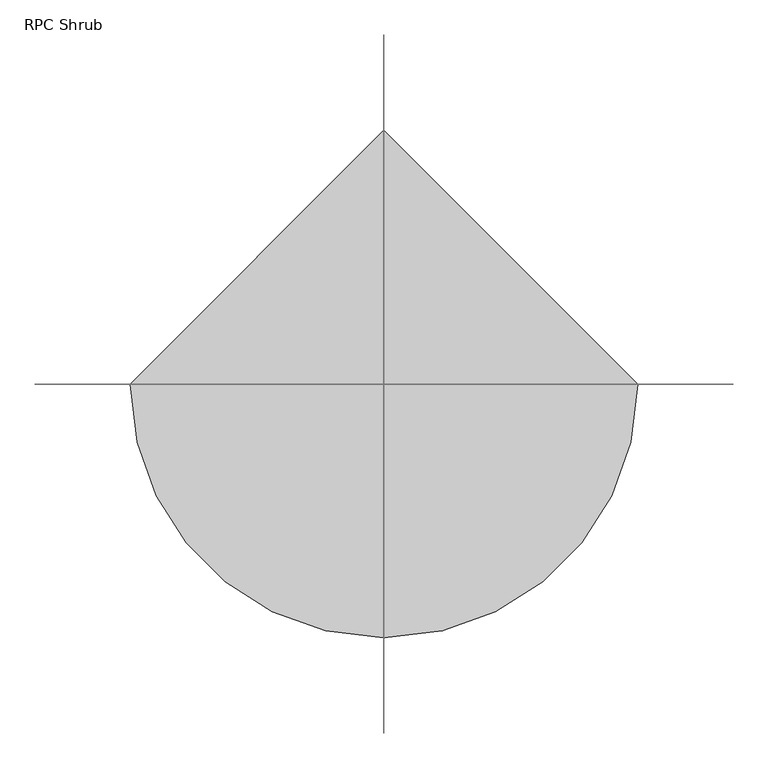
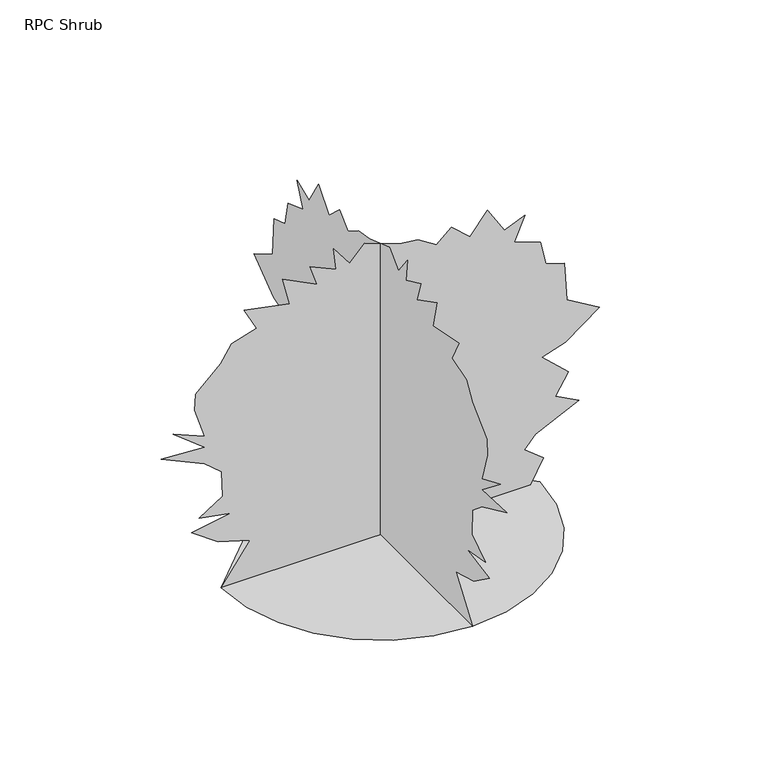
"""IFC4 building model written with IfcOpenShell, lengths in millimetres: geographic element geometry, RPC Shrub."""

from ifc_helpers import new_model, si_unit, origin, place, context, project, spatial, triangles, source, transform, mapped, element, save


def rpc_shrub_d2795376(model_context):
    return source(origin(), model_context, "Body", "Tessellation", [
        triangles([(-812.5409557, 0.0, 3.62e-05), (-791.0601448, -186.180478, 3.62e-05), (-729.8816843, -357.1570149, 3.62e-05), (-633.9078186, -508.0330164, 3.62e-05), (-508.0330164, -633.9078186, 3.62e-05), (-357.1570149, -729.8816843, 3.62e-05), (-186.180478, -791.0601448, 3.62e-05), (3.55e-05, -812.5409557, 3.62e-05), (186.180478, -791.0601448, 3.62e-05), (357.1570149, -729.8816843, 3.62e-05), (508.0330164, -633.9078186, 3.62e-05), (633.9078186, -508.0330164, 3.62e-05), (729.8816843, -357.1570149, 3.62e-05), (791.0601448, -186.180478, 3.62e-05), (812.5409557, 7.1e-05, 3.62e-05), (-0.0001066, 812.5409557, 3.62e-05), (-0.0042747, -811.2988804, 0.0001209), (-0.0042708, -665.7314575, 204.5081021), (-0.004267, -827.9002653, 251.4511125), (-0.004262, -964.4608252, 349.6055863), (-0.004264, -763.884696, 383.7457263), (-0.0042607, -926.0535038, 413.6186849), (-0.0042602, -806.5617422, 490.4333639), (-0.0042562, -810.8289963, 622.7267424), (-0.0042527, -896.1805452, 695.2767471), (-0.0042464, -1118.0927267, 797.697167), (-0.0042501, -896.1805452, 784.8930067), (-0.0042438, -1058.3468822, 912.9192038), (-0.0042483, -896.1805452, 844.6389238), (-0.0042428, -947.3895561, 1002.5380068), (-0.0042404, -943.1223021, 1087.8896284), (-0.0042387, -815.0961777, 1207.38139), (-0.0042368, -759.6175146, 1297.000193), (-0.0042376, -631.5913176, 1335.4075871), (-0.0042331, -695.6044161, 1454.899276), (-0.0042379, -465.1578355, 1407.9550484), (-0.0042331, -499.2979754, 1553.0525871), (-0.0042384, -324.3300579, 1463.4336388), (-0.0042347, -358.4701979, 1570.1213127), (-0.0042384, -226.1755659, 1510.3753956), (-0.0042348, -238.9781819, 1625.6000484), (-0.0042392, -157.8947773, 1518.9123745), (-0.0042379, -81.0790899, 1599.9941986), (-0.0042425, 98.1577894, 1535.9812454), (-0.0042443, 192.0433106, 1523.1795559), (-0.0042475, 285.9303487, 1463.4336388), (-0.0042466, 362.7450096, 1531.7139187), (-0.0042505, 456.6310304, 1446.3622971), (-0.0042486, 546.2498697, 1557.3197685), (-0.0042539, 631.6014914, 1420.7592087), (-0.0042542, 738.2890926, 1463.4336388), (-0.0042571, 682.8104296, 1339.6747684), (-0.0042604, 815.1063515, 1292.7303955), (-0.0042647, 844.9766939, 1164.7042711), (-0.004267, 938.862751, 1134.8313852), (-0.0042731, 951.6669113, 934.2577269), (-0.0042786, 1118.1003571, 836.1044884), (-0.0042798, 943.1324759, 708.078364), (-0.0042791, 823.6407143, 669.67097), (-0.004285, 960.2012741, 541.6448456), (-0.0042871, 891.9209942, 434.9546645), (-0.0042908, 1011.4127558, 370.9416023), (-0.0042907, 789.5005743, 264.2539829), (-0.0042918, 734.0219112, 200.2406482), (-0.0042955, 832.1751497, 123.4246974), (-0.0042982, 766.4170269, 0.0205859), (-811.3090542, 0.0043453, 0.0), (-665.7416313, 0.0043331, 204.5081021), (-827.9078957, 0.0043303, 251.4511125), (-964.4684555, 0.0043245, 349.6055863), (-763.8948698, 0.0043224, 383.7457263), (-926.0611341, 0.0043206, 413.6186849), (-806.5693726, 0.0043161, 490.4333639), (-810.836554, 0.0043082, 622.7267424), (-896.1881756, 0.0043039, 695.2742037), (-1118.1003571, 0.0042978, 797.697167), (-896.1881756, 0.0042985, 784.8930067), (-1058.3545126, 0.0042909, 912.9192038), (-896.1881756, 0.004295, 844.6389238), (-947.3996572, 0.0042855, 1002.5380068), (-943.1299324, 0.0042805, 1087.8896284), (-815.1063515, 0.0042733, 1207.38139), (-759.6276157, 0.004268, 1297.000193), (-631.6014914, 0.0042657, 1335.4075871), (-695.6145899, 0.0042586, 1454.899276), (-465.1654295, 0.0042614, 1407.9550484), (-499.3055695, 0.0042527, 1553.0525871), (-324.3376883, 0.0042581, 1463.4336388), (-358.4778282, 0.0042517, 1570.1213127), (-226.1839592, 0.0042553, 1510.3753956), (-238.9868297, 0.0042484, 1625.6000484), (-157.903425, 0.0042548, 1518.9123745), (-81.0877195, 0.0042499, 1599.9941986), (98.1491599, 0.0042537, 1535.9812454), (192.0346629, 0.0042545, 1523.1795559), (285.9201749, 0.0042581, 1463.4336388), (362.7374156, 0.004254, 1531.7139187), (456.6234364, 0.0042591, 1446.3622971), (546.2422394, 0.0042525, 1557.3197685), (631.5913176, 0.0042606, 1420.7565926), (738.2814623, 0.0042581, 1463.4336388), (682.8027992, 0.0042654, 1339.6747684), (815.0961777, 0.0042682, 1292.7303955), (844.9691362, 0.0042759, 1164.7042711), (938.8551207, 0.0042777, 1134.8313852), (951.6567375, 0.0042896, 934.2577269), (1118.0927267, 0.0042955, 836.1044884), (943.1223021, 0.0043031, 708.078364), (823.6305405, 0.0043054, 669.67097), (960.1936438, 0.004313, 541.6448456), (891.9133638, 0.0043194, 434.9546645), (1011.402582, 0.0043232, 370.9416023), (789.4904005, 0.0043296, 264.2539829), (734.0142809, 0.0043334, 200.2403938), (832.1675194, 0.0043379, 123.4246974), (766.4094692, 0.0043453, 0.020512)], [[15, 16, 1], [14, 15, 1], [14, 1, 2], [13, 14, 2], [13, 2, 3], [13, 3, 4], [12, 13, 4], [11, 12, 4], [11, 4, 5], [11, 5, 6], [11, 6, 7], [11, 7, 8], [11, 8, 9], [11, 9, 10], [27, 28, 29], [25, 26, 27], [40, 41, 42], [21, 22, 23], [50, 51, 52], [19, 20, 21], [38, 39, 40], [36, 37, 38], [34, 35, 36], [61, 62, 63], [66, 17, 18], [56, 57, 58], [48, 49, 50], [18, 19, 21], [46, 47, 48], [64, 65, 66], [59, 60, 61], [56, 58, 59], [54, 55, 56], [42, 43, 44], [52, 53, 54], [54, 56, 59], [24, 25, 27], [48, 50, 52], [59, 61, 63], [52, 54, 59], [48, 52, 59], [46, 48, 59], [66, 18, 21], [30, 31, 32], [29, 30, 32], [66, 21, 23], [66, 23, 24], [64, 66, 24], [63, 64, 24], [59, 63, 24], [46, 59, 24], [45, 46, 24], [44, 45, 24], [42, 44, 24], [40, 42, 24], [38, 40, 24], [36, 38, 24], [34, 36, 24], [34, 24, 27], [34, 27, 29], [34, 29, 32], [33, 34, 32], [77, 78, 79], [75, 76, 77], [90, 91, 92], [71, 72, 73], [100, 101, 102], [69, 70, 71], [88, 89, 90], [86, 87, 88], [84, 85, 86], [111, 112, 113], [116, 67, 68], [106, 107, 108], [98, 99, 100], [68, 69, 71], [96, 97, 98], [114, 115, 116], [109, 110, 111], [106, 108, 109], [104, 105, 106], [92, 93, 94], [102, 103, 104], [104, 106, 109], [74, 75, 77], [98, 100, 102], [109, 111, 113], [102, 104, 109], [98, 102, 109], [96, 98, 109], [116, 68, 71], [80, 81, 82], [79, 80, 82], [116, 71, 73], [116, 73, 74], [114, 116, 74], [113, 114, 74], [109, 113, 74], [96, 109, 74], [95, 96, 74], [94, 95, 74], [92, 94, 74], [90, 92, 74], [88, 90, 74], [86, 88, 74], [84, 86, 74], [84, 74, 77], [84, 77, 79], [84, 79, 82], [83, 84, 82]], closed=False),
    ])


if __name__ == "__main__":
    model = new_model("IFC4")
    model_context = context("Model", 3, world=origin())
    ifc_project = project(units=[si_unit("LENGTHUNIT", "METRE", prefix="MILLI")], contexts=[model_context])
    site = spatial("IfcSite", under=ifc_project)
    building = spatial("IfcBuilding", under=site)
    placement = place(None, origin())
    rpc_shrub_shape = rpc_shrub_d2795376(model_context)
    element("IfcGeographicElement", 1, ObjectType="RPC Shrub", at=placement, inside=building, context=model_context, shape_type="MappedRepresentation", body=[
        mapped(rpc_shrub_shape, transform((0.0, 0.0, 0.0), x_axis=(1.0, 0.0, 0.0), y_axis=(0.0, 1.0, 0.0), z_axis=(0.0, 0.0, 1.0))),
    ])
    save(model, "model.ifc")

# Revit data of these elements
# Type "RPC Shrub"
#   built-in parameter 1005198 = "{2, 15},{39, RPC-16-G3GJ-A6PX-PK1P-U000-ST1L-LVER-AU},{1, 0},{1, 0},{2, 13},{1, 8},{5, Color},{1, 0},{1, 0},{3, 0.8},{3, 0.8},{3, 0.8},{1, 8},{7, BBoxMin},{1, 0},{1, 0},{1, 0},{1, 0},{1, 0},{1, 8},{7, BBoxMax},{1, 0},{1, 0},{1, 0},{1, 0},{1, 0},{2, 11},{9, RPCTypeId},{1, 0},{1, 0},{39, RPC-16-G3GJ-A6PX-PK1P-U000-ST1L-LVER-AU},{1, 6},{14, RPCPlantHeight},{1, 0},{1, 0},{7, 5.33333},{2, 11},{7, keyword},{1, 0},{1, 0},{35, :RPCs:Shrubs & Grasses:Geometry:RPC},{2, 11},{8, category},{1, 0},{1, 0},{16, Shrubs & Grasses},{2, 11},{12, LocalizedUID},{1, 0},{1, 0},{8, Oleander},{2, 14},{6, Height},{1, 0},{1, 0},{7, 5.33333},{1, 2},{16, Cast Reflections},{1, 0},{1, 0},{1, 0},{1, 2},{12, Cast Shadows},{1, 0},{1, 0},{1, 1},{1, 2},{9, Lock View},{1, 0},{1, 0},{1, 0},{1, 4},{5, ViewC},{1, 0},{1, 0},{1, 0},{21, assetlibrary_base.fbx},{1, 5},"
#   built-in parameter 1005195 = "RPC-16-G3GJ-A6PX-PK1P-U000-ST1L-LVER-AU"
#   Assembly Code = "G2050500"
#   Height = 5' - 4"
#   Default Elevation = 0
